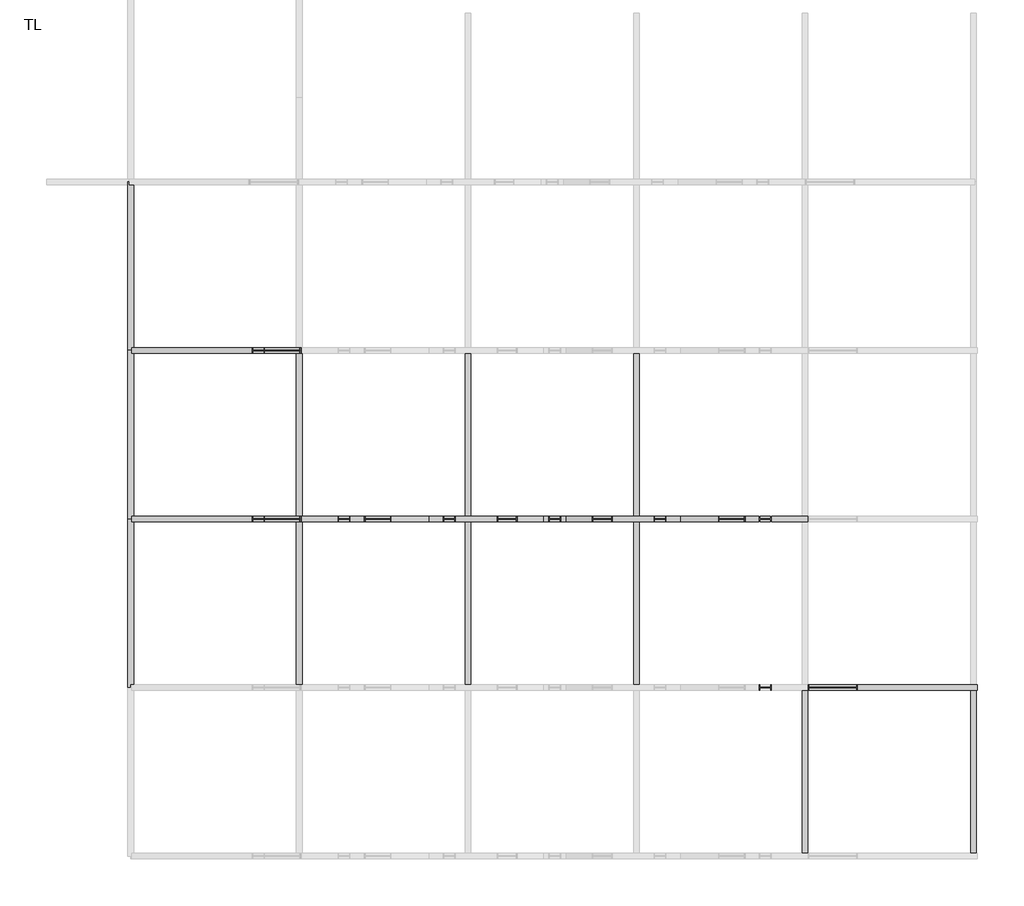
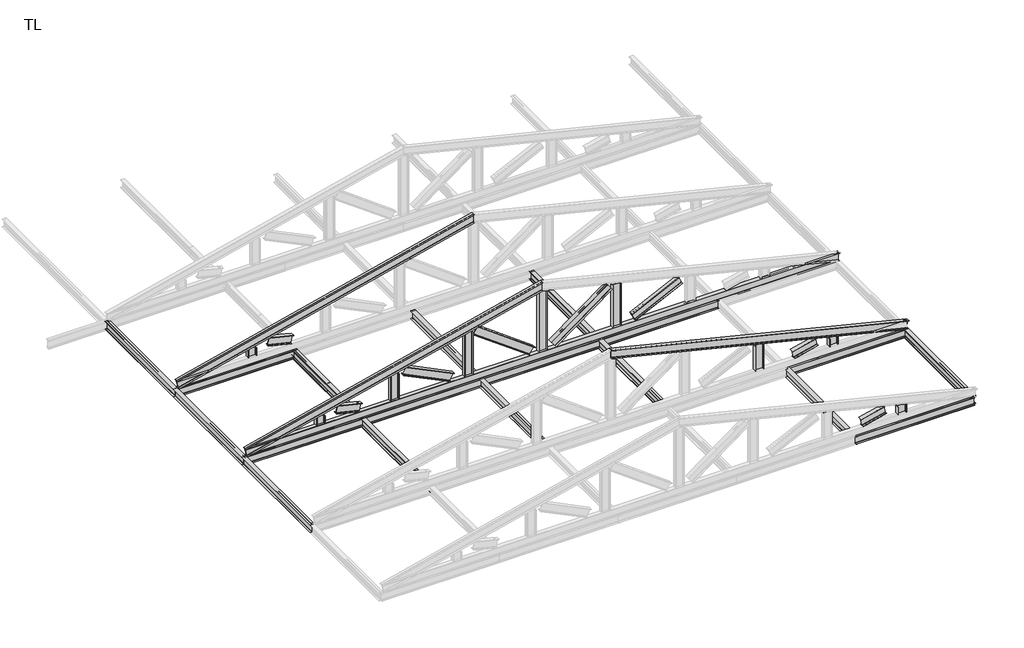
# One storey, part 2 of 4: 39 beams.
"""IFC4 building model written with IfcOpenShell, lengths in millimetres."""

from ifc_helpers import new_model, si_unit, frame, origin, place, context, project, spatial, polyline, circle_curve, ellipse_curve, transform, mapped, element, save
from ifc_brep_helpers import plane_surface, revolved_surface, advanced_brep
from components import w_shapes_w14x30_920474df, w_shapes_w14x30_f0ef5163, w_shapes_w14x30_e8a2e8cf, w_shapes_w14x30_72b19b1b, w_shapes_w14x30_b44ec7f2, w_shapes_w14x30_809da129, w_shapes_w14x30_b6c746c8, w_shapes_w14x30_333ad3b1, w_shapes_w14x30_a113fbeb, w_shapes_w14x30_23e28ad8, w_shapes_w14x30_8f152a7c, w_shapes_w14x30_95bb247d

model = new_model("IFC4")

# Units and contexts
model_context = context("Model", 3, world=origin())
ifc_project = project(units=[si_unit("LENGTHUNIT", "METRE", prefix="MILLI")], contexts=[model_context])

# Site, building, storey
site = spatial("IfcSite", under=ifc_project)
building = spatial("IfcBuilding", under=site)
storey = spatial("IfcBuildingStorey", under=building, Name="TL", Elevation=8534.4)

# Beams
placement = place(None, origin())
element("IfcBeam", 1, ObjectType="W Shapes : W14X30", at=placement, inside=storey, context=model_context, shape_type="AdvancedBrep", body=[
    advanced_brep(
    [(-18310.2356148, 9124.3335479, 8538.7295322), (-18307.9189802, 9124.3335479, 8529.2288983), (-18307.9189802, 8953.3915479, 8529.2288983), (-18310.2356148, 8953.3915479, 8538.7295322), (-18310.2356148, 9025.2735479, 8538.7295322), (-18312.6425079, 9035.4335479, 8548.6003207), (-18386.2332635, 9035.4335479, 8850.3996793), (-18388.6401565, 9025.2735479, 8860.2704678), (-18388.6401565, 8953.3915479, 8860.2704678), (-18390.9567911, 8953.3915479, 8869.7711017), (-18390.9567911, 9124.3335479, 8869.7711017), (-18388.6401565, 9124.3335479, 8860.2704678), (-18388.6401565, 9052.4515479, 8860.2704678), (-18386.2332635, 9042.2915479, 8850.3996793), (-18312.6425079, 9042.2915479, 8548.6003207), (-18310.2356148, 9052.4515479, 8538.7295322), (-5849.4378857, 9052.4515479, 11577.1704505), (-5849.4378857, 9124.3335479, 11577.1704505), (-5849.4378857, 9042.2915479, 11587.6281358), (-5849.4378857, 9042.2915479, 11907.3718642), (-5849.4378857, 9052.4515479, 11917.8295495), (-5849.4378857, 9124.3335479, 11917.8295495), (-5849.4378857, 9124.3335479, 11927.8950717), (-5849.4378857, 8953.3915479, 11927.8950717), (-5849.4378857, 8953.3915479, 11917.8295495), (-5849.4378857, 9025.2735479, 11917.8295495), (-5849.4378857, 9035.4335479, 11907.3718642), (-5849.4378857, 9035.4335479, 11587.6281358), (-5849.4378857, 9025.2735479, 11577.1704505), (-5849.4378857, 8953.3915479, 11577.1704505), (-5849.4378857, 8953.3915479, 11567.1049283), (-5849.4378857, 9124.3335479, 11567.1049283)],
    [
        (0, 1),
        (1, 2),
        (2, 3),
        (3, 4),
        (4, 5, circle_curve(frame((-18312.6425079, 9025.2735479, 8548.6003207), z_axis=(0.971534301878756, 0.0, 0.23689892417011604), x_axis=(0.23689892417011604, 0.0, -0.971534301878756)), 10.16)),
        (5, 6),
        (6, 7, circle_curve(frame((-18386.2332635, 9025.2735479, 8850.3996793), z_axis=(0.971534301878756, 0.0, 0.23689892417011604), x_axis=(0.0, 1.0000000000000002, 0.0)), 10.16)),
        (7, 8),
        (8, 9),
        (9, 10),
        (10, 11),
        (11, 12),
        (12, 13, circle_curve(frame((-18386.2332635, 9052.4515479, 8850.3996793), z_axis=(0.971534301878756, 0.0, 0.23689892417011604), x_axis=(-0.23689892417011604, 0.0, 0.971534301878756)), 10.16)),
        (13, 14),
        (14, 15, circle_curve(frame((-18312.6425079, 9052.4515479, 8548.6003207), z_axis=(0.971534301878756, 0.0, 0.23689892417011604), x_axis=(0.0, -1.0000000000000002, 0.0)), 10.16)),
        (15, 0),
        (16, 17),
        (17, 0),
        (15, 16),
        (18, 16, ellipse_curve(frame((-5849.4378857, 9052.4515479, 11587.6281358), z_axis=(1.0, 0.0, 0.0), x_axis=(0.0, 0.0, -1.0)), 10.4576853, 10.16)),
        (14, 18),
        (19, 18),
        (13, 19),
        (20, 19, ellipse_curve(frame((-5849.4378857, 9052.4515479, 11907.3718642), z_axis=(1.0, 0.0, 0.0), x_axis=(0.0, 0.0, -1.0)), 10.4576853, 10.16)),
        (12, 20),
        (21, 20),
        (11, 21),
        (22, 21),
        (10, 22),
        (23, 22),
        (9, 23),
        (24, 23),
        (8, 24),
        (25, 24),
        (7, 25),
        (26, 25, ellipse_curve(frame((-5849.4378857, 9025.2735479, 11907.3718642), z_axis=(1.0, 0.0, 0.0), x_axis=(0.0, 0.0, -1.0)), 10.4576853, 10.16)),
        (6, 26),
        (27, 26),
        (5, 27),
        (28, 27, ellipse_curve(frame((-5849.4378857, 9025.2735479, 11587.6281358), z_axis=(1.0, 0.0, 0.0), x_axis=(0.0, 0.0, -1.0)), 10.4576853, 10.16)),
        (4, 28),
        (29, 28),
        (3, 29),
        (30, 29),
        (2, 30),
        (31, 30),
        (1, 31),
        (17, 31),
    ],
    [
        plane_surface(frame((-18349.4378857, 9038.8625479, 8699.5), z_axis=(-0.971534301878756, 0.0, -0.23689892417011604), x_axis=(-0.23689892417011604, 0.0, 0.971534301878756))),
        plane_surface(frame((-5810.2356148, 9088.3925479, 11586.7295322), z_axis=(-0.23689892417011604, 0.0, 0.971534301878756), x_axis=(0.0, -1.0, 0.0))),
        revolved_surface(polyline([(-18312.6425079, 9042.2915479, 8548.600320699998), (-5847.030992628227, 9042.2915479, 11588.215032583868)]), (-5812.6425079, 9052.4515479, 11596.6003207), (-0.971534301878756, 0.0, -0.23689892417011604)),
        plane_surface(frame((-5849.4378857, 9042.2915479, 11747.5), z_axis=(0.0, 1.0000000000000002, 0.0), x_axis=(-0.23689892417011604, 0.0, 0.971534301878756))),
        revolved_surface(polyline([(-18388.640156569567, 9052.4515479, 8860.270467807088), (-5849.437885708268, 9052.4515479, 11917.82954953391)]), (-5886.2332635, 9052.4515479, 11898.3996793), (-0.971534301878756, 0.0, -0.23689892417011604)),
        plane_surface(frame((-5888.6401565, 9088.3925479, 11908.2704678), z_axis=(0.23689892417011604, 0.0, -0.971534301878756), x_axis=(0.0, 1.0, 0.0))),
        plane_surface(frame((-5889.7984738, 9124.3335479, 11913.0207848), z_axis=(0.0, 1.0000000000000002, 0.0), x_axis=(-0.23689892417011604, 0.0, 0.971534301878756))),
        plane_surface(frame((-5890.9567911, 9038.8625479, 11917.7711017), z_axis=(-0.23689892417011604, 0.0, 0.971534301878756), x_axis=(0.0, -1.0, 0.0))),
        plane_surface(frame((-5889.7984738, 8953.3915479, 11913.0207848), z_axis=(0.0, -1.0000000000000002, 0.0), x_axis=(0.23689892417011604, 0.0, -0.971534301878756))),
        plane_surface(frame((-5888.6401565, 8989.3325479, 11908.2704678), z_axis=(0.23689892417011604, 0.0, -0.971534301878756), x_axis=(0.0, 1.0, 0.0))),
        revolved_surface(polyline([(-18386.2332635, 9035.4335479, 8850.399679299999), (-5847.0309926387, 9035.4335479, 11907.95876102682)]), (-5886.2332635, 9025.2735479, 11898.3996793), (-0.971534301878756, 0.0, -0.23689892417011604)),
        plane_surface(frame((-5849.4378857, 9035.4335479, 11747.5), z_axis=(0.0, -1.0000000000000002, 0.0), x_axis=(0.23689892417011604, 0.0, -0.971534301878756))),
        revolved_surface(polyline([(-18310.23561483043, 9025.2735479, 8538.729532192909), (-5844.624099558659, 9025.2735479, 11578.34424407678)]), (-5812.6425079, 9025.2735479, 11596.6003207), (-0.971534301878756, 0.0, -0.23689892417011604)),
        plane_surface(frame((-5810.2356148, 8989.3325479, 11586.7295322), z_axis=(-0.23689892417011604, 0.0, 0.971534301878756), x_axis=(0.0, -1.0, 0.0))),
        plane_surface(frame((-5809.0772975, 8953.3915479, 11581.9792152), z_axis=(0.0, -1.0000000000000002, 0.0), x_axis=(0.23689892417011604, 0.0, -0.971534301878756))),
        plane_surface(frame((-5807.9189802, 9038.8625479, 11577.2288983), z_axis=(0.23689892417011604, 0.0, -0.971534301878756), x_axis=(0.0, 1.0, 0.0))),
        plane_surface(frame((-5809.0772975, 9124.3335479, 11581.9792152), z_axis=(0.0, 1.0000000000000002, 0.0), x_axis=(-0.23689892417011604, 0.0, 0.971534301878756))),
        plane_surface(frame((-5849.4378857, 9038.8625479, 11927.8950717), z_axis=(1.0, 0.0, 0.0), x_axis=(0.0, -1.0, 0.0))),
    ],
    [
        (0, [[1, 2, 3, 4, 5, 6, 7, 8, 9, 10, 11, 12, 13, 14, 15, 16]]),
        (1, [[17, 18, -16, 19]]),
        (2, [[20, -19, -15, 21]]),
        (3, [[22, -21, -14, 23]]),
        (4, [[24, -23, -13, 25]]),
        (5, [[26, -25, -12, 27]]),
        (6, [[28, -27, -11, 29]]),
        (7, [[30, -29, -10, 31]]),
        (8, [[32, -31, -9, 33]]),
        (9, [[34, -33, -8, 35]]),
        (10, [[36, -35, -7, 37]]),
        (11, [[38, -37, -6, 39]]),
        (12, [[40, -39, -5, 41]]),
        (13, [[42, -41, -4, 43]]),
        (14, [[44, -43, -3, 45]]),
        (15, [[46, -45, -2, 47]]),
        (16, [[48, -47, -1, -18]]),
        (17, [[-17, -20, -22, -24, -26, -28, -30, -32, -34, -36, -38, -40, -42, -44, -46, -48]]),
    ],
),
])
element("IfcBeam", 2, ObjectType="W Shapes : W14X30", at=placement, inside=storey, context=model_context, shape_type="AdvancedBrep", body=[
    advanced_brep(
    [(-18310.2356148, 4124.3335479, 8538.7295322), (-18307.9189802, 4124.3335479, 8529.2288983), (-18307.9189802, 3953.3915479, 8529.2288983), (-18310.2356148, 3953.3915479, 8538.7295322), (-18310.2356148, 4025.2735479, 8538.7295322), (-18312.6425079, 4035.4335479, 8548.6003207), (-18386.2332635, 4035.4335479, 8850.3996793), (-18388.6401565, 4025.2735479, 8860.2704678), (-18388.6401565, 3953.3915479, 8860.2704678), (-18390.9567911, 3953.3915479, 8869.7711017), (-18390.9567911, 4124.3335479, 8869.7711017), (-18388.6401565, 4124.3335479, 8860.2704678), (-18388.6401565, 4052.4515479, 8860.2704678), (-18386.2332635, 4042.2915479, 8850.3996793), (-18312.6425079, 4042.2915479, 8548.6003207), (-18310.2356148, 4052.4515479, 8538.7295322), (-5849.4378857, 4052.4515479, 11577.1704505), (-5849.4378857, 4124.3335479, 11577.1704505), (-5849.4378857, 4042.2915479, 11587.6281358), (-5849.4378857, 4042.2915479, 11907.3718642), (-5849.4378857, 4052.4515479, 11917.8295495), (-5849.4378857, 4124.3335479, 11917.8295495), (-5849.4378857, 4124.3335479, 11927.8950717), (-5849.4378857, 3953.3915479, 11927.8950717), (-5849.4378857, 3953.3915479, 11917.8295495), (-5849.4378857, 4025.2735479, 11917.8295495), (-5849.4378857, 4035.4335479, 11907.3718642), (-5849.4378857, 4035.4335479, 11587.6281358), (-5849.4378857, 4025.2735479, 11577.1704505), (-5849.4378857, 3953.3915479, 11577.1704505), (-5849.4378857, 3953.3915479, 11567.1049283), (-5849.4378857, 4124.3335479, 11567.1049283)],
    [
        (0, 1),
        (1, 2),
        (2, 3),
        (3, 4),
        (4, 5, circle_curve(frame((-18312.6425079, 4025.2735479, 8548.6003207), z_axis=(0.971534301878756, 0.0, 0.23689892417011604), x_axis=(0.23689892417011604, 0.0, -0.971534301878756)), 10.16)),
        (5, 6),
        (6, 7, circle_curve(frame((-18386.2332635, 4025.2735479, 8850.3996793), z_axis=(0.971534301878756, 0.0, 0.23689892417011604), x_axis=(0.0, 1.0000000000000002, 0.0)), 10.16)),
        (7, 8),
        (8, 9),
        (9, 10),
        (10, 11),
        (11, 12),
        (12, 13, circle_curve(frame((-18386.2332635, 4052.4515479, 8850.3996793), z_axis=(0.971534301878756, 0.0, 0.23689892417011604), x_axis=(-0.23689892417011604, 0.0, 0.971534301878756)), 10.16)),
        (13, 14),
        (14, 15, circle_curve(frame((-18312.6425079, 4052.4515479, 8548.6003207), z_axis=(0.971534301878756, 0.0, 0.23689892417011604), x_axis=(0.0, -1.0000000000000002, 0.0)), 10.16)),
        (15, 0),
        (16, 17),
        (17, 0),
        (15, 16),
        (18, 16, ellipse_curve(frame((-5849.4378857, 4052.4515479, 11587.6281358), z_axis=(1.0, 0.0, 0.0), x_axis=(0.0, 0.0, -1.0)), 10.4576853, 10.16)),
        (14, 18),
        (19, 18),
        (13, 19),
        (20, 19, ellipse_curve(frame((-5849.4378857, 4052.4515479, 11907.3718642), z_axis=(1.0, 0.0, 0.0), x_axis=(0.0, 0.0, -1.0)), 10.4576853, 10.16)),
        (12, 20),
        (21, 20),
        (11, 21),
        (22, 21),
        (10, 22),
        (23, 22),
        (9, 23),
        (24, 23),
        (8, 24),
        (25, 24),
        (7, 25),
        (26, 25, ellipse_curve(frame((-5849.4378857, 4025.2735479, 11907.3718642), z_axis=(1.0, 0.0, 0.0), x_axis=(0.0, 0.0, -1.0)), 10.4576853, 10.16)),
        (6, 26),
        (27, 26),
        (5, 27),
        (28, 27, ellipse_curve(frame((-5849.4378857, 4025.2735479, 11587.6281358), z_axis=(1.0, 0.0, 0.0), x_axis=(0.0, 0.0, -1.0)), 10.4576853, 10.16)),
        (4, 28),
        (29, 28),
        (3, 29),
        (30, 29),
        (2, 30),
        (31, 30),
        (1, 31),
        (17, 31),
    ],
    [
        plane_surface(frame((-18349.4378857, 4038.8625479, 8699.5), z_axis=(-0.971534301878756, 0.0, -0.23689892417011604), x_axis=(-0.23689892417011604, 0.0, 0.971534301878756))),
        plane_surface(frame((-5810.2356148, 4088.3925479, 11586.7295322), z_axis=(-0.23689892417011604, 0.0, 0.971534301878756), x_axis=(0.0, -1.0, 0.0))),
        revolved_surface(polyline([(-18312.6425079, 4042.2915479000003, 8548.600320699998), (-5847.030992628227, 4042.2915479000003, 11588.215032583868)]), (-5812.6425079, 4052.4515479, 11596.6003207), (-0.971534301878756, 0.0, -0.23689892417011604)),
        plane_surface(frame((-5849.4378857, 4042.2915479, 11747.5), z_axis=(0.0, 1.0000000000000002, 0.0), x_axis=(-0.23689892417011604, 0.0, 0.971534301878756))),
        revolved_surface(polyline([(-18388.640156569567, 4052.4515479, 8860.270467807088), (-5849.437885708268, 4052.4515479, 11917.82954953391)]), (-5886.2332635, 4052.4515479, 11898.3996793), (-0.971534301878756, 0.0, -0.23689892417011604)),
        plane_surface(frame((-5888.6401565, 4088.3925479, 11908.2704678), z_axis=(0.23689892417011604, 0.0, -0.971534301878756), x_axis=(0.0, 1.0, 0.0))),
        plane_surface(frame((-5889.7984738, 4124.3335479, 11913.0207848), z_axis=(0.0, 1.0000000000000002, 0.0), x_axis=(-0.23689892417011604, 0.0, 0.971534301878756))),
        plane_surface(frame((-5890.9567911, 4038.8625479, 11917.7711017), z_axis=(-0.23689892417011604, 0.0, 0.971534301878756), x_axis=(0.0, -1.0, 0.0))),
        plane_surface(frame((-5889.7984738, 3953.3915479, 11913.0207848), z_axis=(0.0, -1.0000000000000002, 0.0), x_axis=(0.23689892417011604, 0.0, -0.971534301878756))),
        plane_surface(frame((-5888.6401565, 3989.3325479, 11908.2704678), z_axis=(0.23689892417011604, 0.0, -0.971534301878756), x_axis=(0.0, 1.0, 0.0))),
        revolved_surface(polyline([(-18386.2332635, 4035.4335478999997, 8850.399679299999), (-5847.0309926387, 4035.4335478999997, 11907.95876102682)]), (-5886.2332635, 4025.2735479, 11898.3996793), (-0.971534301878756, 0.0, -0.23689892417011604)),
        plane_surface(frame((-5849.4378857, 4035.4335479, 11747.5), z_axis=(0.0, -1.0000000000000002, 0.0), x_axis=(0.23689892417011604, 0.0, -0.971534301878756))),
        revolved_surface(polyline([(-18310.23561483043, 4025.2735479, 8538.729532192909), (-5844.624099558659, 4025.2735479, 11578.34424407678)]), (-5812.6425079, 4025.2735479, 11596.6003207), (-0.971534301878756, 0.0, -0.23689892417011604)),
        plane_surface(frame((-5810.2356148, 3989.3325479, 11586.7295322), z_axis=(-0.23689892417011604, 0.0, 0.971534301878756), x_axis=(0.0, -1.0, 0.0))),
        plane_surface(frame((-5809.0772975, 3953.3915479, 11581.9792152), z_axis=(0.0, -1.0000000000000002, 0.0), x_axis=(0.23689892417011604, 0.0, -0.971534301878756))),
        plane_surface(frame((-5807.9189802, 4038.8625479, 11577.2288983), z_axis=(0.23689892417011604, 0.0, -0.971534301878756), x_axis=(0.0, 1.0, 0.0))),
        plane_surface(frame((-5809.0772975, 4124.3335479, 11581.9792152), z_axis=(0.0, 1.0000000000000002, 0.0), x_axis=(-0.23689892417011604, 0.0, 0.971534301878756))),
        plane_surface(frame((-5849.4378857, 4038.8625479, 11927.8950717), z_axis=(1.0, 0.0, 0.0), x_axis=(0.0, -1.0, 0.0))),
    ],
    [
        (0, [[1, 2, 3, 4, 5, 6, 7, 8, 9, 10, 11, 12, 13, 14, 15, 16]]),
        (1, [[17, 18, -16, 19]]),
        (2, [[20, -19, -15, 21]]),
        (3, [[22, -21, -14, 23]]),
        (4, [[24, -23, -13, 25]]),
        (5, [[26, -25, -12, 27]]),
        (6, [[28, -27, -11, 29]]),
        (7, [[30, -29, -10, 31]]),
        (8, [[32, -31, -9, 33]]),
        (9, [[34, -33, -8, 35]]),
        (10, [[36, -35, -7, 37]]),
        (11, [[38, -37, -6, 39]]),
        (12, [[40, -39, -5, 41]]),
        (13, [[42, -41, -4, 43]]),
        (14, [[44, -43, -3, 45]]),
        (15, [[46, -45, -2, 47]]),
        (16, [[48, -47, -1, -18]]),
        (17, [[-17, -20, -22, -24, -26, -28, -30, -32, -34, -36, -38, -40, -42, -44, -46, -48]]),
    ],
),
])
element("IfcBeam", 3, ObjectType="W Shapes : W14X30", at=placement, inside=storey, context=model_context, shape_type="AdvancedBrep", body=[
    advanced_brep(
    [(6611.3598435, -875.6664521, 8538.7295322), (6611.3598435, -947.5484521, 8538.7295322), (6613.7667365, -957.7084521, 8548.6003207), (6687.3574921, -957.7084521, 8850.3996793), (6689.7643852, -947.5484521, 8860.2704678), (6689.7643852, -875.6664521, 8860.2704678), (6692.0810198, -875.6664521, 8869.7711017), (6692.0810198, -1046.6084521, 8869.7711017), (6689.7643852, -1046.6084521, 8860.2704678), (6689.7643852, -974.7264521, 8860.2704678), (6687.3574921, -964.5664521, 8850.3996793), (6613.7667365, -964.5664521, 8548.6003207), (6611.3598435, -974.7264521, 8538.7295322), (6611.3598435, -1046.6084521, 8538.7295322), (6609.0432089, -1046.6084521, 8529.2288983), (6609.0432089, -875.6664521, 8529.2288983), (-5849.4378857, -875.6664521, 11577.1704505), (-5849.4378857, -947.5484521, 11577.1704505), (-5849.4378857, -957.7084521, 11587.6281358), (-5849.4378857, -957.7084521, 11907.3718642), (-5849.4378857, -947.5484521, 11917.8295495), (-5849.4378857, -875.6664521, 11917.8295495), (-5849.4378857, -875.6664521, 11927.8950717), (-5849.4378857, -1046.6084521, 11927.8950717), (-5849.4378857, -1046.6084521, 11917.8295495), (-5849.4378857, -974.7264521, 11917.8295495), (-5849.4378857, -964.5664521, 11907.3718642), (-5849.4378857, -964.5664521, 11587.6281358), (-5849.4378857, -974.7264521, 11577.1704505), (-5849.4378857, -1046.6084521, 11577.1704505), (-5849.4378857, -1046.6084521, 11567.1049283), (-5849.4378857, -875.6664521, 11567.1049283)],
    [
        (0, 1),
        (1, 2, circle_curve(frame((6613.7667365, -947.5484521, 8548.6003207), z_axis=(-0.971534301878756, 0.0, 0.23689892417011588), x_axis=(0.0, -1.0, 0.0)), 10.16)),
        (2, 3),
        (3, 4, circle_curve(frame((6687.3574921, -947.5484521, 8850.3996793), z_axis=(-0.971534301878756, 0.0, 0.23689892417011588), x_axis=(0.23689892417011588, 0.0, 0.971534301878756)), 10.16)),
        (4, 5),
        (5, 6),
        (6, 7),
        (7, 8),
        (8, 9),
        (9, 10, circle_curve(frame((6687.3574921, -974.7264521, 8850.3996793), z_axis=(-0.971534301878756, 0.0, 0.23689892417011588), x_axis=(0.0, 1.0, 0.0)), 10.16)),
        (10, 11),
        (11, 12, circle_curve(frame((6613.7667365, -974.7264521, 8548.6003207), z_axis=(-0.971534301878756, 0.0, 0.23689892417011588), x_axis=(-0.23689892417011588, 0.0, -0.971534301878756)), 10.16)),
        (12, 13),
        (13, 14),
        (14, 15),
        (15, 0),
        (0, 16),
        (16, 17),
        (17, 1),
        (17, 18, ellipse_curve(frame((-5849.4378857, -947.5484521, 11587.6281358), z_axis=(-1.0, 0.0, 0.0), x_axis=(0.0, 0.0, 1.0)), 10.4576853, 10.16)),
        (18, 2),
        (18, 19),
        (19, 3),
        (19, 20, ellipse_curve(frame((-5849.4378857, -947.5484521, 11907.3718642), z_axis=(-1.0, 0.0, 0.0), x_axis=(0.0, 0.0, 1.0)), 10.4576853, 10.16)),
        (20, 4),
        (20, 21),
        (21, 5),
        (21, 22),
        (22, 6),
        (22, 23),
        (23, 7),
        (23, 24),
        (24, 8),
        (24, 25),
        (25, 9),
        (25, 26, ellipse_curve(frame((-5849.4378857, -974.7264521, 11907.3718642), z_axis=(-1.0, 0.0, 0.0), x_axis=(0.0, 0.0, 1.0)), 10.4576853, 10.16)),
        (26, 10),
        (26, 27),
        (27, 11),
        (27, 28, ellipse_curve(frame((-5849.4378857, -974.7264521, 11587.6281358), z_axis=(-1.0, 0.0, 0.0), x_axis=(0.0, 0.0, 1.0)), 10.4576853, 10.16)),
        (28, 12),
        (28, 29),
        (29, 13),
        (29, 30),
        (30, 14),
        (30, 31),
        (31, 15),
        (31, 16),
    ],
    [
        plane_surface(frame((6650.5621143, -961.1374521, 8699.5), z_axis=(0.971534301878756, 0.0, -0.23689892417011588), x_axis=(0.23689892417011588, 0.0, 0.971534301878756))),
        plane_surface(frame((6611.3598435, -911.6074521, 8538.7295322), z_axis=(0.23689892417011588, 0.0, 0.971534301878756), x_axis=(0.0, -1.0, 0.0))),
        revolved_surface(polyline([(-5851.844778771774, -957.7084520999999, 11588.215032583868), (6613.766736564033, -957.7084520999999, 8548.600320684385)]), (6613.7667365, -947.5484521, 8548.6003207), (-0.971534301878756, 0.0, 0.23689892417011588)),
        plane_surface(frame((6650.5621143, -957.7084521, 8699.5), z_axis=(0.0, 1.0, 0.0), x_axis=(0.23689892417011588, 0.0, 0.971534301878756))),
        revolved_surface(polyline([(-5849.437885691734, -947.5484521, 11917.82954953391), (6689.764385199924, -947.5484521, 8860.270467799688)]), (6687.3574921, -947.5484521, 8850.3996793), (-0.971534301878756, 0.0, 0.23689892417011588)),
        plane_surface(frame((6689.7643852, -911.6074521, 8860.2704678), z_axis=(-0.23689892417011588, 0.0, -0.971534301878756), x_axis=(0.0, 1.0, 0.0))),
        plane_surface(frame((6690.9227025, -875.6664521, 8865.0207848), z_axis=(0.0, 1.0, 0.0), x_axis=(0.23689892417011588, 0.0, 0.971534301878756))),
        plane_surface(frame((6692.0810198, -961.1374521, 8869.7711017), z_axis=(0.23689892417011588, 0.0, 0.971534301878756), x_axis=(0.0, -1.0, 0.0))),
        plane_surface(frame((6690.9227025, -1046.6084521, 8865.0207848), z_axis=(0.0, -1.0, 0.0), x_axis=(-0.23689892417011588, 0.0, -0.971534301878756))),
        plane_surface(frame((6689.7643852, -1010.6674521, 8860.2704678), z_axis=(-0.23689892417011588, 0.0, -0.971534301878756), x_axis=(0.0, 1.0, 0.0))),
        revolved_surface(polyline([(-5851.844778761302, -964.5664521, 11907.95876102682), (6687.357492130355, -964.5664521, 8850.3996792926)]), (6687.3574921, -974.7264521, 8850.3996793), (-0.971534301878756, 0.0, 0.23689892417011588)),
        plane_surface(frame((6650.5621143, -964.5664521, 8699.5), z_axis=(0.0, -1.0, 0.0), x_axis=(-0.23689892417011588, 0.0, -0.971534301878756))),
        revolved_surface(polyline([(-5854.251671841343, -974.7264521, 11578.34424407678), (6611.359843494464, -974.7264521, 8538.729532177296)]), (6613.7667365, -974.7264521, 8548.6003207), (-0.971534301878756, 0.0, 0.23689892417011588)),
        plane_surface(frame((6611.3598435, -1010.6674521, 8538.7295322), z_axis=(0.23689892417011588, 0.0, 0.971534301878756), x_axis=(0.0, -1.0, 0.0))),
        plane_surface(frame((6610.2015262, -1046.6084521, 8533.9792152), z_axis=(0.0, -1.0, 0.0), x_axis=(-0.23689892417011588, 0.0, -0.971534301878756))),
        plane_surface(frame((6609.0432089, -961.1374521, 8529.2288983), z_axis=(-0.23689892417011588, 0.0, -0.971534301878756), x_axis=(0.0, 1.0, 0.0))),
        plane_surface(frame((6610.2015262, -875.6664521, 8533.9792152), z_axis=(0.0, 1.0, 0.0), x_axis=(0.23689892417011588, 0.0, 0.971534301878756))),
        plane_surface(frame((-5849.4378857, -961.1374521, 11927.8950717), z_axis=(-1.0, 0.0, 0.0), x_axis=(0.0, 1.0, 0.0))),
    ],
    [
        (0, [[1, 2, 3, 4, 5, 6, 7, 8, 9, 10, 11, 12, 13, 14, 15, 16]]),
        (1, [[-1, 17, 18, 19]]),
        (2, [[-2, -19, 20, 21]]),
        (3, [[-3, -21, 22, 23]]),
        (4, [[-4, -23, 24, 25]]),
        (5, [[-5, -25, 26, 27]]),
        (6, [[-6, -27, 28, 29]]),
        (7, [[-7, -29, 30, 31]]),
        (8, [[-8, -31, 32, 33]]),
        (9, [[-9, -33, 34, 35]]),
        (10, [[-10, -35, 36, 37]]),
        (11, [[-11, -37, 38, 39]]),
        (12, [[-12, -39, 40, 41]]),
        (13, [[-13, -41, 42, 43]]),
        (14, [[-14, -43, 44, 45]]),
        (15, [[-15, -45, 46, 47]]),
        (16, [[-16, -47, 48, -17]]),
        (17, [[-48, -46, -44, -42, -40, -38, -36, -34, -32, -30, -28, -26, -24, -22, -20, -18]]),
    ],
),
])
w_shapes_w14x30_shape = w_shapes_w14x30_920474df(model_context)
element("IfcBeam", 4, ObjectType="W Shapes : W14X30", at=placement, inside=storey, context=model_context, shape_type="MappedRepresentation", body=[
    mapped(w_shapes_w14x30_shape, transform((4074.3621143, -5961.1374521, 8359.14), x_axis=(1.0, 0.0, 0.0), y_axis=(0.0, 1.0, 0.0), z_axis=(0.0, 0.0, 1.0))),
])
element("IfcBeam", 5, ObjectType="W Shapes : W14X30", at=placement, inside=storey, context=model_context, shape_type="MappedRepresentation", body=[
    mapped(w_shapes_w14x30_shape, transform((4074.3621143, -961.1374521, 8359.14), x_axis=(1.0, 0.0, 0.0), y_axis=(0.0, 1.0, 0.0), z_axis=(0.0, 0.0, 1.0))),
])
element("IfcBeam", 6, ObjectType="W Shapes : W14X30", at=placement, inside=storey, context=model_context, shape_type="MappedRepresentation", body=[
    mapped(w_shapes_w14x30_shape, transform((-15925.6378857, 4038.8625479, 8359.14), x_axis=(1.0, 0.0, 0.0), y_axis=(0.0, 1.0, 0.0), z_axis=(0.0, 0.0, 1.0))),
])
element("IfcBeam", 7, ObjectType="W Shapes : W14X30", at=placement, inside=storey, context=model_context, shape_type="MappedRepresentation", body=[
    mapped(w_shapes_w14x30_shape, transform((-10925.6378857, 4038.8625479, 8359.14), x_axis=(1.0, 0.0, 0.0), y_axis=(0.0, 1.0, 0.0), z_axis=(0.0, 0.0, 1.0))),
])
element("IfcBeam", 8, ObjectType="W Shapes : W14X30", at=placement, inside=storey, context=model_context, shape_type="MappedRepresentation", body=[
    mapped(w_shapes_w14x30_shape, transform((-5925.6378857, 4038.8625479, 8359.14), x_axis=(1.0, 0.0, 0.0), y_axis=(0.0, 1.0, 0.0), z_axis=(0.0, 0.0, 1.0))),
])
element("IfcBeam", 9, ObjectType="W Shapes : W14X30", at=placement, inside=storey, context=model_context, shape_type="MappedRepresentation", body=[
    mapped(w_shapes_w14x30_shape, transform((-925.6378857, 4038.8625479, 8359.14), x_axis=(1.0, 0.0, 0.0), y_axis=(0.0, 1.0, 0.0), z_axis=(0.0, 0.0, 1.0))),
])
element("IfcBeam", 10, ObjectType="W Shapes : W14X30", at=placement, inside=storey, context=model_context, shape_type="MappedRepresentation", body=[
    mapped(w_shapes_w14x30_shape, transform((-15925.6378857, 9038.8625479, 8359.14), x_axis=(1.0, 0.0, 0.0), y_axis=(0.0, 1.0, 0.0), z_axis=(0.0, 0.0, 1.0))),
])
element("IfcBeam", 11, ObjectType="W Shapes : W14X30", at=placement, inside=storey, context=model_context, shape_type="MappedRepresentation", body=[
    mapped(w_shapes_w14x30_shape, transform((6574.3621143, -3461.1374521, 8359.14), x_axis=(0.0, 1.0, 0.0), y_axis=(-1.0, 0.0, 0.0), z_axis=(0.0, 0.0, 1.0))),
])
element("IfcBeam", 12, ObjectType="W Shapes : W14X30", at=placement, inside=storey, context=model_context, shape_type="MappedRepresentation", body=[
    mapped(w_shapes_w14x30_shape, transform((1574.3621143, -3461.1374521, 8359.14), x_axis=(0.0, 1.0, 0.0), y_axis=(-1.0, 0.0, 0.0), z_axis=(0.0, 0.0, 1.0))),
])
element("IfcBeam", 13, ObjectType="W Shapes : W14X30", at=placement, inside=storey, context=model_context, shape_type="MappedRepresentation", body=[
    mapped(w_shapes_w14x30_shape, transform((-3425.6378857, 1538.8625479, 8359.14), x_axis=(0.0, 1.0, 0.0), y_axis=(-1.0, 0.0, 0.0), z_axis=(0.0, 0.0, 1.0))),
])
element("IfcBeam", 14, ObjectType="W Shapes : W14X30", at=placement, inside=storey, context=model_context, shape_type="MappedRepresentation", body=[
    mapped(w_shapes_w14x30_shape, transform((-3425.6378857, 6538.8625479, 8359.14), x_axis=(0.0, 1.0, 0.0), y_axis=(-1.0, 0.0, 0.0), z_axis=(0.0, 0.0, 1.0))),
])
element("IfcBeam", 15, ObjectType="W Shapes : W14X30", at=placement, inside=storey, context=model_context, shape_type="MappedRepresentation", body=[
    mapped(w_shapes_w14x30_shape, transform((-8425.6378857, 1538.8625479, 8359.14), x_axis=(0.0, 1.0, 0.0), y_axis=(-1.0, 0.0, 0.0), z_axis=(0.0, 0.0, 1.0))),
])
element("IfcBeam", 16, ObjectType="W Shapes : W14X30", at=placement, inside=storey, context=model_context, shape_type="MappedRepresentation", body=[
    mapped(w_shapes_w14x30_shape, transform((-8425.6378857, 6538.8625479, 8359.14), x_axis=(0.0, 1.0, 0.0), y_axis=(-1.0, 0.0, 0.0), z_axis=(0.0, 0.0, 1.0))),
])
element("IfcBeam", 17, ObjectType="W Shapes : W14X30", at=placement, inside=storey, context=model_context, shape_type="MappedRepresentation", body=[
    mapped(w_shapes_w14x30_shape, transform((-13425.6378857, 1538.8625479, 8359.14), x_axis=(0.0, 1.0, 0.0), y_axis=(-1.0, 0.0, 0.0), z_axis=(0.0, 0.0, 1.0))),
])
element("IfcBeam", 18, ObjectType="W Shapes : W14X30", at=placement, inside=storey, context=model_context, shape_type="MappedRepresentation", body=[
    mapped(w_shapes_w14x30_shape, transform((-13425.6378857, 6538.8625479, 8359.14), x_axis=(0.0, 1.0, 0.0), y_axis=(-1.0, 0.0, 0.0), z_axis=(0.0, 0.0, 1.0))),
])
element("IfcBeam", 19, ObjectType="W Shapes : W14X30", at=placement, inside=storey, context=model_context, shape_type="MappedRepresentation", body=[
    mapped(w_shapes_w14x30_shape, transform((-18425.6378857, 1538.8625479, 8359.14), x_axis=(0.0, 1.0, 0.0), y_axis=(-1.0, 0.0, 0.0), z_axis=(0.0, 0.0, 1.0))),
])
element("IfcBeam", 20, ObjectType="W Shapes : W14X30", at=placement, inside=storey, context=model_context, shape_type="MappedRepresentation", body=[
    mapped(w_shapes_w14x30_shape, transform((-18425.6378857, 6538.8625479, 8359.14), x_axis=(0.0, 1.0, 0.0), y_axis=(-1.0, 0.0, 0.0), z_axis=(0.0, 0.0, 1.0))),
])
element("IfcBeam", 21, ObjectType="W Shapes : W14X30", at=placement, inside=storey, context=model_context, shape_type="MappedRepresentation", body=[
    mapped(w_shapes_w14x30_shape, transform((-18425.6378857, 11538.8625479, 8359.14), x_axis=(0.0, 1.0, 0.0), y_axis=(-1.0, 0.0, 0.0), z_axis=(0.0, 0.0, 1.0))),
])
w_shapes_w14x30_2_shape = w_shapes_w14x30_f0ef5163(model_context)
element("IfcBeam", 22, ObjectType="W Shapes : W14X30", at=placement, inside=storey, context=model_context, shape_type="MappedRepresentation", body=[
    mapped(w_shapes_w14x30_2_shape, transform((-5849.4378857, 4038.8625479, 8699.5), x_axis=(1.0, 0.0, 0.0), y_axis=(0.0, 1.0, 0.0), z_axis=(0.0, 0.0, 1.0))),
])
w_shapes_w14x30_3_shape = w_shapes_w14x30_e8a2e8cf(model_context)
element("IfcBeam", 23, ObjectType="W Shapes : W14X30", at=placement, inside=storey, context=model_context, shape_type="MappedRepresentation", body=[
    mapped(w_shapes_w14x30_3_shape, transform((-5849.4378857, 4038.8625479, 10223.5), x_axis=(0.0, 0.0, 1.0), y_axis=(0.0, -1.0, 0.0), z_axis=(1.0, 0.0, 0.0))),
])
w_shapes_w14x30_4_shape = w_shapes_w14x30_72b19b1b(model_context)
element("IfcBeam", 24, ObjectType="W Shapes : W14X30", at=placement, inside=storey, context=model_context, shape_type="MappedRepresentation", body=[
    mapped(w_shapes_w14x30_4_shape, transform((-8974.4378857, 4038.8625479, 9842.5), x_axis=(0.0, 0.0, 1.0), y_axis=(0.0, -1.0, 0.0), z_axis=(1.0, 0.0, 0.0))),
])
element("IfcBeam", 25, ObjectType="W Shapes : W14X30", at=placement, inside=storey, context=model_context, shape_type="MappedRepresentation", body=[
    mapped(w_shapes_w14x30_4_shape, transform((-2724.4378857, 4038.8625479, 9842.5), x_axis=(0.0, 0.0, 1.0), y_axis=(0.0, -1.0, 0.0), z_axis=(1.0, 0.0, 0.0))),
])
w_shapes_w14x30_5_shape = w_shapes_w14x30_b44ec7f2(model_context)
element("IfcBeam", 26, ObjectType="W Shapes : W14X30", at=placement, inside=storey, context=model_context, shape_type="MappedRepresentation", body=[
    mapped(w_shapes_w14x30_5_shape, transform((-12099.4378857, 4038.8625479, 9461.5), x_axis=(0.0, 0.0, 1.0), y_axis=(0.0, -1.0, 0.0), z_axis=(1.0, 0.0, 0.0))),
])
element("IfcBeam", 27, ObjectType="W Shapes : W14X30", at=placement, inside=storey, context=model_context, shape_type="MappedRepresentation", body=[
    mapped(w_shapes_w14x30_5_shape, transform((400.5621143, -961.1374521, 9461.5), x_axis=(0.0, 0.0, 1.0), y_axis=(0.0, -1.0, 0.0), z_axis=(1.0, 0.0, 0.0))),
])
w_shapes_w14x30_6_shape = w_shapes_w14x30_809da129(model_context)
element("IfcBeam", 28, ObjectType="W Shapes : W14X30", at=placement, inside=storey, context=model_context, shape_type="MappedRepresentation", body=[
    mapped(w_shapes_w14x30_6_shape, transform((-15224.4378857, 9038.8625479, 9080.5), x_axis=(0.0, 0.0, 1.0), y_axis=(0.0, -1.0, 0.0), z_axis=(1.0, 0.0, 0.0))),
])
element("IfcBeam", 29, ObjectType="W Shapes : W14X30", at=placement, inside=storey, context=model_context, shape_type="MappedRepresentation", body=[
    mapped(w_shapes_w14x30_6_shape, transform((-15224.4378857, 4038.8625479, 9080.5), x_axis=(0.0, 0.0, 1.0), y_axis=(0.0, -1.0, 0.0), z_axis=(1.0, 0.0, 0.0))),
])
element("IfcBeam", 30, ObjectType="W Shapes : W14X30", at=placement, inside=storey, context=model_context, shape_type="MappedRepresentation", body=[
    mapped(w_shapes_w14x30_6_shape, transform((3525.5621143, -961.1374521, 9080.5), x_axis=(0.0, 0.0, 1.0), y_axis=(0.0, -1.0, 0.0), z_axis=(1.0, 0.0, 0.0))),
])
element("IfcBeam", 31, ObjectType="W Shapes : W14X30", at=placement, inside=storey, context=model_context, shape_type="MappedRepresentation", body=[
    mapped(w_shapes_w14x30_6_shape, transform((3525.5621143, -5961.1374521, 9080.5), x_axis=(0.0, 0.0, 1.0), y_axis=(0.0, -1.0, 0.0), z_axis=(1.0, 0.0, 0.0))),
])
w_shapes_w14x30_7_shape = w_shapes_w14x30_b6c746c8(model_context)
element("IfcBeam", 32, ObjectType="W Shapes : W14X30", at=placement, inside=storey, context=model_context, shape_type="MappedRepresentation", body=[
    mapped(w_shapes_w14x30_7_shape, transform((-7411.9378857, 4038.8625479, 9842.5), x_axis=(0.8071023678442881, 0.0, -0.5904115241254555), y_axis=(0.0, -1.0, 0.0), z_axis=(-0.5904115241254555, 0.0, -0.8071023678442881))),
])
w_shapes_w14x30_8_shape = w_shapes_w14x30_333ad3b1(model_context)
element("IfcBeam", 33, ObjectType="W Shapes : W14X30", at=placement, inside=storey, context=model_context, shape_type="MappedRepresentation", body=[
    mapped(w_shapes_w14x30_8_shape, transform((-10536.9378857, 4038.8625479, 9461.5), x_axis=(0.8988126690463005, 0.0, -0.4383329624405008), y_axis=(0.0, -1.0, 0.0), z_axis=(-0.4383329624405008, 0.0, -0.8988126690463005))),
])
w_shapes_w14x30_9_shape = w_shapes_w14x30_a113fbeb(model_context)
element("IfcBeam", 34, ObjectType="W Shapes : W14X30", at=placement, inside=storey, context=model_context, shape_type="MappedRepresentation", body=[
    mapped(w_shapes_w14x30_9_shape, transform((-4286.9378857, 4038.8625479, 9842.5), x_axis=(0.8071023678442877, 0.0, 0.590411524125456), y_axis=(0.0, -1.0, 0.0), z_axis=(0.590411524125456, 0.0, -0.8071023678442877))),
])
w_shapes_w14x30_10_shape = w_shapes_w14x30_23e28ad8(model_context)
element("IfcBeam", 35, ObjectType="W Shapes : W14X30", at=placement, inside=storey, context=model_context, shape_type="MappedRepresentation", body=[
    mapped(w_shapes_w14x30_10_shape, transform((-1161.9378857, 4038.8625479, 9461.5), x_axis=(0.8988126690463014, 0.0, 0.4383329624404991), y_axis=(0.0, -1.0, 0.0), z_axis=(0.4383329624404991, 0.0, -0.8988126690463014))),
])
w_shapes_w14x30_11_shape = w_shapes_w14x30_8f152a7c(model_context)
element("IfcBeam", 36, ObjectType="W Shapes : W14X30", at=placement, inside=storey, context=model_context, shape_type="MappedRepresentation", body=[
    mapped(w_shapes_w14x30_11_shape, transform((-13661.9378857, 9038.8625479, 9080.5), x_axis=(0.9715343018787559, 0.0, -0.23689892417011585), y_axis=(0.0, -1.0, 0.0), z_axis=(-0.23689892417011585, 0.0, -0.9715343018787559))),
])
element("IfcBeam", 37, ObjectType="W Shapes : W14X30", at=placement, inside=storey, context=model_context, shape_type="MappedRepresentation", body=[
    mapped(w_shapes_w14x30_11_shape, transform((-13661.9378857, 4038.8625479, 9080.5), x_axis=(0.9715343018787559, 0.0, -0.23689892417011585), y_axis=(0.0, -1.0, 0.0), z_axis=(-0.23689892417011585, 0.0, -0.9715343018787559))),
])
w_shapes_w14x30_12_shape = w_shapes_w14x30_95bb247d(model_context)
element("IfcBeam", 38, ObjectType="W Shapes : W14X30", at=placement, inside=storey, context=model_context, shape_type="MappedRepresentation", body=[
    mapped(w_shapes_w14x30_12_shape, transform((1963.0621143, -961.1374521, 9080.5), x_axis=(0.971534301878756, 0.0, 0.2368989241701152), y_axis=(0.0, -1.0, 0.0), z_axis=(0.2368989241701152, 0.0, -0.971534301878756))),
])
element("IfcBeam", 39, ObjectType="W Shapes : W14X30", at=placement, inside=storey, context=model_context, shape_type="MappedRepresentation", body=[
    mapped(w_shapes_w14x30_12_shape, transform((1963.0621143, -5961.1374521, 9080.5), x_axis=(0.971534301878756, 0.0, 0.2368989241701152), y_axis=(0.0, -1.0, 0.0), z_axis=(0.2368989241701152, 0.0, -0.971534301878756))),
])

save(model, "model.ifc")

# Revit data of these elements
# Type "W Shapes : W14X30"
#   Section Name Key = "W14X30"
#   Width = 6.730"
#   Web Thickness = 0.270"
#   Web Fillet = 0.400"
#   Warping Constant = 887.00 in⁶
#   Torsional Moment of Inertia = 0.38 in⁴
#   Section Area = 8.85 in²
#   Plastic Modulus weak axis = 8.99 in³
#   Plastic Modulus strong axis = 47.30 in³
#   Perimeter = 4.441 ft²/ft
#   Nominal Weight = 30.00 lbf/ft
#   Moment of Inertia weak axis = 19.60 in⁴
#   Moment of Inertia strong axis = 291.00 in⁴
#   Height = 13.800"
#   Flange Thickness = 0.385"
#   Elastic Modulus weak axis = 5.82 in³
#   Elastic Modulus strong axis = 42.00 in³
#   Clear Web Height = 0' - 11 5/8"
#   Centroid Vertical = 6.900"
#   Centroid Horizontal = 3.365"
#   Bolt Spacing = 0' - 3 1/2"
#   Length [instance default] = 1524 mm
#   Structural Material [instance default] = Steel ASTM A992
#   Principal Axes Angle = 0
# Elements 1, 2, 3 (IfcBeam, "W Shapes : W14X30")
#   Length = 12866.247 mm
#   Structural Material = Steel ASTM A992
#   Phase Created = New Construction
#   Materials on its faces: "Steel ASTM A992"
# Elements 4, 5, 6, 7, 8, 9, 10, 11, 12, 13, 14, 15, 16, 17, 18, 19, 20, 21 (IfcBeam, "W Shapes : W14X30")
#   Length = 5000 mm
#   Structural Material = Steel ASTM A992
#   Phase Created = New Construction
#   Materials on its faces: "Steel ASTM A992"
# Element 22 (IfcBeam, "W Shapes : W14X30")
#   Length = 25000 mm
#   Structural Material = Steel ASTM A992
#   Phase Created = New Construction
#   Materials on its faces: "Steel ASTM A992"
# Element 23 (IfcBeam, "W Shapes : W14X30")
#   Length = 3048 mm
#   Structural Material = Steel ASTM A992
#   Phase Created = New Construction
#   Materials on its faces: "Steel ASTM A992"
# Elements 24, 25 (IfcBeam, "W Shapes : W14X30")
#   Length = 2286 mm
#   Structural Material = Steel ASTM A992
#   Phase Created = New Construction
#   Materials on its faces: "Steel ASTM A992"
# Elements 26, 27 (IfcBeam, "W Shapes : W14X30")
#   Length = 1524 mm
#   Structural Material = Steel ASTM A992
#   Phase Created = New Construction
#   Materials on its faces: "Steel ASTM A992"
# Elements 28, 29, 30, 31 (IfcBeam, "W Shapes : W14X30")
#   Length = 762 mm
#   Structural Material = Steel ASTM A992
#   Phase Created = New Construction
#   Materials on its faces: "Steel ASTM A992"
# Elements 32, 34 (IfcBeam, "W Shapes : W14X30")
#   Length = 3871.876 mm
#   Structural Material = Steel ASTM A992
#   Phase Created = New Construction
#   Materials on its faces: "Steel ASTM A992"
# Elements 33, 35 (IfcBeam, "W Shapes : W14X30")
#   Length = 3476.809 mm
#   Structural Material = Steel ASTM A992
#   Phase Created = New Construction
#   Materials on its faces: "Steel ASTM A992"
# Elements 36, 37, 38, 39 (IfcBeam, "W Shapes : W14X30")
#   Length = 3216.562 mm
#   Structural Material = Steel ASTM A992
#   Phase Created = New Construction
#   Materials on its faces: "Steel ASTM A992"
# Materials
#   "Steel ASTM A992": class "Metal", colour RGB 199 199 199, transparency 0, Description = "Structural steel 50ksi", Cost = 0
